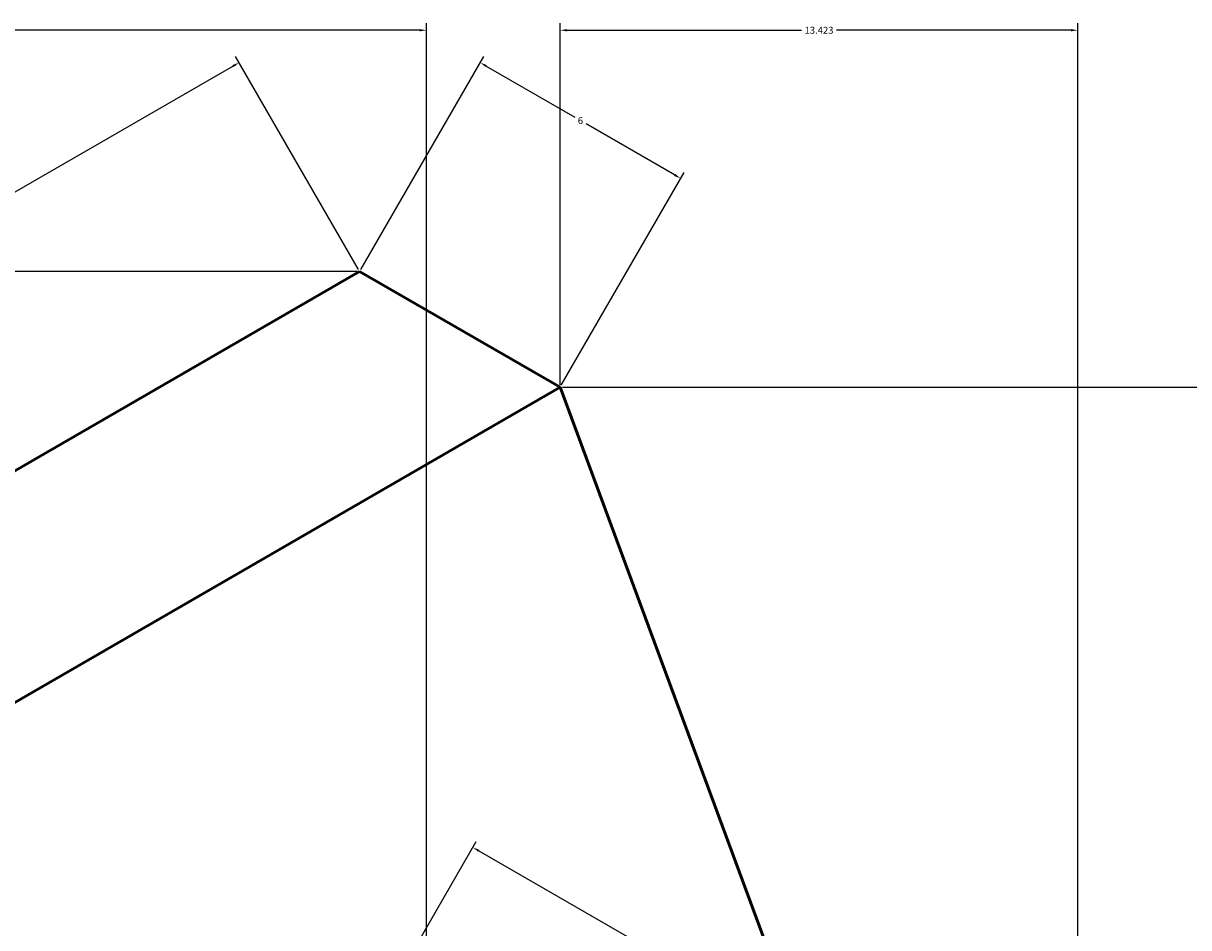
# Model space of a CAD drawing. Units: inches. Extents: x -23 to 69, y -27 to 96.
# Tile 9 of 10: x 7 to 37, y 72 to 96. Entities that reach past the tile are written whole.
import ezdxf

# ---------------------------------------------------------------- set-up
doc = ezdxf.new("R2010")
doc.units = ezdxf.units.IN
doc.header["$MEASUREMENT"] = 0
doc.layers.add('M-DIMS', color=2, linetype='Continuous', lineweight=18)
doc.layers.add('M-OUTL', color=7, linetype='Continuous', lineweight=50)
doc.styles.get("Standard").update_dxf_attribs({"font": 'arial.ttf'})
doc.dimstyles.get("Standard").update_dxf_attribs({"dimtxt": 0.18, "dimasz": 0.18, "dimexe": 0.18, "dimexo": 0.0625, "dimgap": 0.09, "dimtad": 0, "dimtih": 1, "dimtoh": 1, "dimdec": 4, "dimzin": 0, "dimdsep": 46, "dimtxsty": 'Standard', "dimcen": 0.09, "dimadec": 0, "dimazin": 0, "dimtfac": 1, "dimtdec": 4, "dimtofl": 0, "dimtmove": 0, "dimatfit": 3, "dimfxl": 1, "dimtolj": 1, "dimtzin": 0, "dimarcsym": 0})

# ---------------------------------------------------------------- blocks, each defined once
blk = doc.blocks.new('*D8')
at = {"layer": 'Defpoints', "color": 0, "transparency": 16777216}
for p in [(12.713, 94.531), (15.838, 89.119), (-13.607, 72.119)]:
    blk.add_point(p, dxfattribs=at)
at = {"layer": 'M-DIMS', "color": 0, "lineweight": -2, "transparency": 16777216}
for p, q in [((15.807, 89.173), (12.623, 94.687)), ((12.557, 94.441), (-1.791, 86.157)), ((-16.576, 77.621), (-2.228, 85.905)), ((-13.638, 72.173), (-16.822, 77.687))]:
    blk.add_line(p, q, dxfattribs=at)
at = {"layer": 'M-DIMS', "color": 0, "transparency": 16777216}
for points in [[(12.542, 94.467), (12.572, 94.415), (12.713, 94.531)], [(-16.591, 77.647), (-16.561, 77.595), (-16.732, 77.531)]]:
    blk.add_solid(points, dxfattribs=at)
at = {"layer": 'M-DIMS', "color": 0, "transparency": 16777216, "insert": (-2.009, 86.031), "char_height": 0.18, "attachment_point": 5}
blk.add_mtext('\\A1;34', dxfattribs=at)
blk = doc.blocks.new('*D9')
at = {"layer": 'Defpoints', "color": 0, "transparency": 16777216}
for p in [(24.159, 91.531), (15.838, 89.119), (21.034, 86.119)]:
    blk.add_point(p, dxfattribs=at)
at = {"layer": 'M-DIMS', "color": 0, "lineweight": -2, "transparency": 16777216}
for p, q in [((15.869, 89.173), (19.053, 94.687)), ((19.119, 94.441), (21.412, 93.118)), ((24.003, 91.621), (21.711, 92.945)), ((21.066, 86.173), (24.249, 91.687))]:
    blk.add_line(p, q, dxfattribs=at)
at = {"layer": 'M-DIMS', "color": 0, "transparency": 16777216}
for points in [[(19.134, 94.467), (19.104, 94.415), (18.963, 94.531)], [(24.018, 91.647), (23.988, 91.595), (24.159, 91.531)]]:
    blk.add_solid(points, dxfattribs=at)
at = {"layer": 'M-DIMS', "color": 0, "transparency": 16777216, "insert": (21.561, 93.031), "char_height": 0.18, "attachment_point": 5}
blk.add_mtext('\\A1;6', dxfattribs=at)
blk = doc.blocks.new('*D10')
at = {"layer": 'Defpoints', "color": 0, "transparency": 16777216}
for p in [(27.431, 69.199), (15.646, 68.786), (24.306, 63.786)]:
    blk.add_point(p, dxfattribs=at)
at = {"layer": 'M-DIMS', "color": 0, "lineweight": -2, "transparency": 16777216}
for p, q in [((15.677, 68.84), (18.861, 74.354)), ((18.927, 74.109), (22.891, 71.82)), ((27.275, 69.289), (23.311, 71.577)), ((24.338, 63.84), (27.521, 69.354))]:
    blk.add_line(p, q, dxfattribs=at)
at = {"layer": 'M-DIMS', "color": 0, "transparency": 16777216}
for points in [[(18.942, 74.135), (18.912, 74.083), (18.771, 74.199)], [(27.29, 69.315), (27.26, 69.263), (27.431, 69.199)]]:
    blk.add_solid(points, dxfattribs=at)
at = {"layer": 'M-DIMS', "color": 0, "transparency": 16777216, "insert": (23.101, 71.699), "char_height": 0.18, "attachment_point": 5}
blk.add_mtext('\\A1;10', dxfattribs=at)
blk = doc.blocks.new('*D13')
at = {"layer": 'Defpoints', "color": 0, "transparency": 16777216}
for p in [(15.838, 89.119), (-22.888, -20.881), (36.623, -20.881)]:
    blk.add_point(p, dxfattribs=at)
at = {"layer": 'M-DIMS', "color": 0, "lineweight": -2, "transparency": 16777216}
for p, q in [((15.776, 89.119), (-23.068, 89.119)), ((-22.888, 88.939), (-22.888, 34.301)), ((-22.888, -20.701), (-22.888, 33.937)), ((36.56, -20.881), (-23.068, -20.881))]:
    blk.add_line(p, q, dxfattribs=at)
at = {"layer": 'M-DIMS', "color": 0, "transparency": 16777216}
for points in [[(-22.918, 88.939), (-22.858, 88.939), (-22.888, 89.119)], [(-22.918, -20.701), (-22.858, -20.701), (-22.888, -20.881)]]:
    blk.add_solid(points, dxfattribs=at)
at = {"layer": 'M-DIMS', "color": 0, "transparency": 16777216, "insert": (-22.888, 34.119), "char_height": 0.18, "attachment_point": 5}
blk.add_mtext('\\A1;110', dxfattribs=at)
blk = doc.blocks.new('*D14')
at = {"layer": 'Defpoints', "color": 0, "transparency": 16777216}
for p in [(21.034, 95.369), (21.034, 86.119), (34.458, 49.869)]:
    blk.add_point(p, dxfattribs=at)
at = {"layer": 'M-DIMS', "color": 0, "lineweight": -2, "transparency": 16777216}
for p, q in [((21.034, 86.181), (21.034, 95.549)), ((34.458, 49.931), (34.458, 95.549)), ((21.214, 95.369), (27.291, 95.369)), ((34.278, 95.369), (28.201, 95.369))]:
    blk.add_line(p, q, dxfattribs=at)
at = {"layer": 'M-DIMS', "color": 0, "transparency": 16777216}
for points in [[(21.214, 95.399), (21.214, 95.339), (21.034, 95.369)], [(34.278, 95.399), (34.278, 95.339), (34.458, 95.369)]]:
    blk.add_solid(points, dxfattribs=at)
at = {"layer": 'M-DIMS', "color": 0, "transparency": 16777216, "insert": (27.746, 95.369), "char_height": 0.18, "attachment_point": 5}
blk.add_mtext('\\A1;13.423', dxfattribs=at)
blk = doc.blocks.new('*D15')
at = {"layer": 'Defpoints', "color": 0, "transparency": 16777216}
for p in [(21.034, 86.119), (68.421, 86.119), (17.57, 52.119)]:
    blk.add_point(p, dxfattribs=at)
at = {"layer": 'M-DIMS', "color": 0, "lineweight": -2, "transparency": 16777216}
for p, q in [((21.097, 86.119), (68.601, 86.119)), ((68.421, 85.939), (68.421, 69.301)), ((68.421, 52.299), (68.421, 68.937)), ((17.633, 52.119), (68.601, 52.119))]:
    blk.add_line(p, q, dxfattribs=at)
at = {"layer": 'M-DIMS', "color": 0, "transparency": 16777216}
for points in [[(68.391, 85.939), (68.451, 85.939), (68.421, 86.119)], [(68.391, 52.299), (68.451, 52.299), (68.421, 52.119)]]:
    blk.add_solid(points, dxfattribs=at)
at = {"layer": 'M-DIMS', "color": 0, "transparency": 16777216, "insert": (68.421, 69.119), "char_height": 0.18, "attachment_point": 5}
blk.add_mtext('\\A1;34', dxfattribs=at)
blk = doc.blocks.new('*D16')
at = {"layer": 'Defpoints', "color": 0, "transparency": 16777216}
for p in [(17.57, 95.369), (-8.41, 69.119), (17.57, 52.119)]:
    blk.add_point(p, dxfattribs=at)
at = {"layer": 'M-DIMS', "color": 0, "lineweight": -2, "transparency": 16777216}
for p, q in [((-8.41, 69.181), (-8.41, 95.549)), ((17.57, 52.181), (17.57, 95.549)), ((-8.23, 95.369), (4.184, 95.369)), ((17.39, 95.369), (4.975, 95.369))]:
    blk.add_line(p, q, dxfattribs=at)
at = {"layer": 'M-DIMS', "color": 0, "transparency": 16777216}
for points in [[(-8.23, 95.399), (-8.23, 95.339), (-8.41, 95.369)], [(17.39, 95.399), (17.39, 95.339), (17.57, 95.369)]]:
    blk.add_solid(points, dxfattribs=at)
at = {"layer": 'M-DIMS', "color": 0, "transparency": 16777216, "insert": (4.58, 95.369), "char_height": 0.18, "attachment_point": 5}
blk.add_mtext('\\A1;25.98', dxfattribs=at)

msp = doc.modelspace()

# ---------------------------------------------------------------- linework, layer by layer
at = {"layer": 'M-OUTL'}
for p, q in [((-13.6066, 72.1186), (15.8382, 89.1186)), ((15.8382, 89.1186), (21.0344, 86.1186)), ((21.0344, 86.1186), (-8.4105, 69.1186)), ((21.0344, 86.1186), (34.4578, 49.8686))]:
    msp.add_line(p, q, dxfattribs=at)

# ---------------------------------------------------------------- dimensions: what is measured, and where the dimension line sits
at = {"layer": 'M-DIMS'}
for base, p1, p2, override, picture, middle in [((17.5703, 95.3686), (-8.4105, 69.1186), (17.5703, 52.1186), {"dimdec": 2, "dimlfac": 1, "dimrnd": 0, "dimzin": 0, "dimdsep": 46, "dimlunit": 2}, '*D16', (4.5799, 95.3686)), ((21.0344, 95.3686), (34.4578, 49.8686), (21.0344, 86.1186), {"dimdec": 3, "dimlfac": 1, "dimrnd": 0, "dimzin": 0, "dimdsep": 46, "dimlunit": 2}, '*D14', (27.7461, 95.3686))]:
    dim = msp.add_linear_dim(base=base, p1=p1, p2=p2, dimstyle='Standard', override=override, dxfattribs=at)
    dim.commit()
    dim.dimension.update_dxf_attribs({"geometry": picture, "text_midpoint": middle})
for base, p1, p2, angle, picture, middle in [((12.7132, 94.5313), (-13.6066, 72.1186), (15.8382, 89.1186), 30, '*D8', (-2.0092, 86.0313)), ((24.1594, 91.5313), (15.8382, 89.1186), (21.0344, 86.1186), 330, '*D9', (21.5613, 93.0313)), ((-22.8877, -20.8814), (15.8382, 89.1186), (36.6228, -20.8814), 90, '*D13', (-22.8877, 34.1186)), ((68.4206, 86.1186), (17.5703, 52.1186), (21.0344, 86.1186), 90, '*D15', (68.4206, 69.1186)), ((27.4314, 69.1986), (15.6461, 68.7859), (24.3064, 63.7859), 330, '*D10', (23.1012, 71.6986))]:
    dim = msp.add_linear_dim(base=base, p1=p1, p2=p2, angle=angle, dimstyle='Standard', override={"dimdec": 0, "dimlfac": 1, "dimrnd": 0, "dimzin": 0, "dimdsep": 46, "dimlunit": 2}, dxfattribs=at)
    dim.commit()
    dim.dimension.update_dxf_attribs({"geometry": picture, "text_midpoint": middle})

doc.saveas('drawing.dxf')
